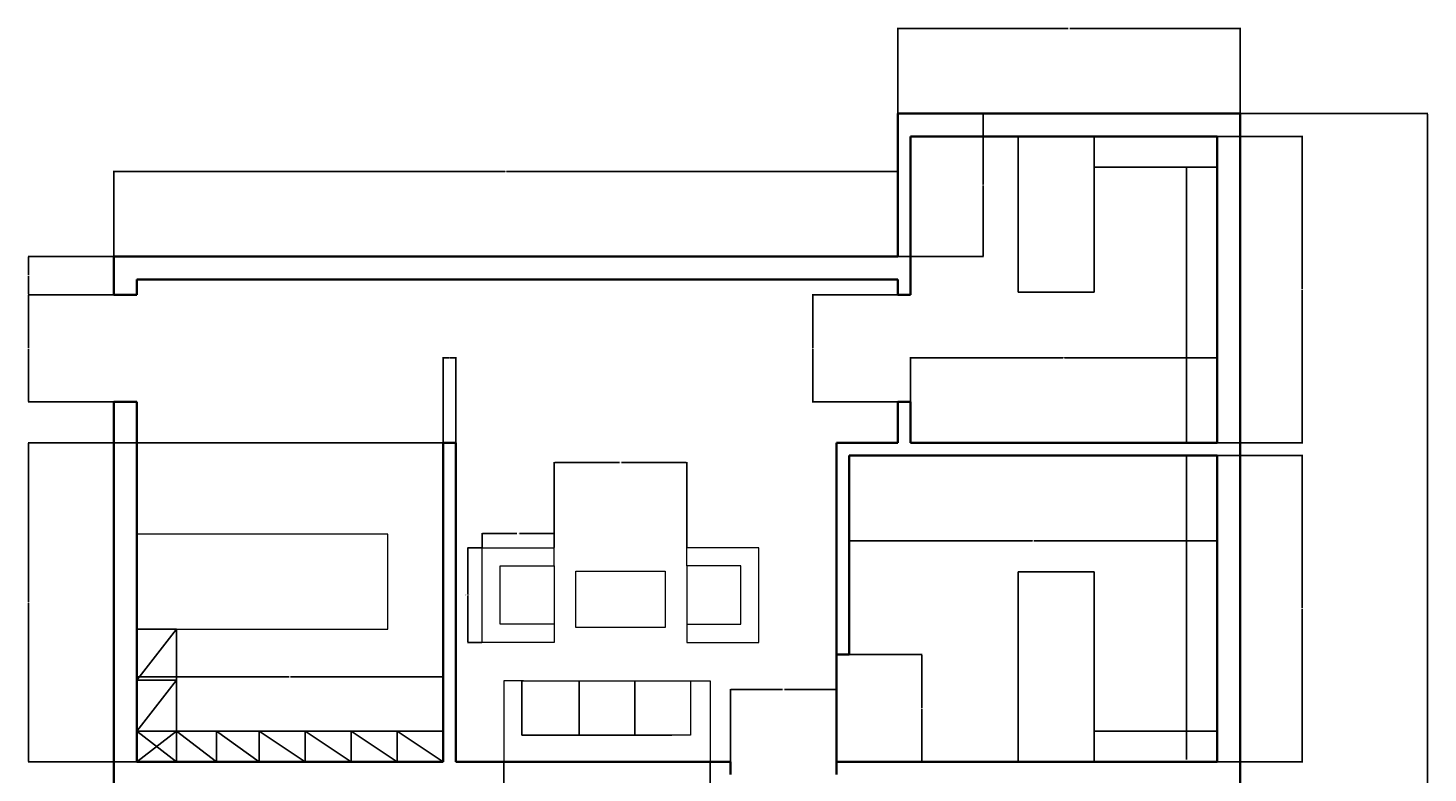
# Model space of a CAD drawing. Units: inches. Extents: x 1201 to 1750, y 1179 to 1858.
# Tile 3 of 3: x 1201 to 1750, y 1566 to 1858. Entities that reach past the tile are written whole.
import ezdxf

# ---------------------------------------------------------------- set-up
doc = ezdxf.new("R2010")
doc.units = ezdxf.units.IN
for name, color, linetype, lineweight in [('A-ANNO-DIMS', 2, 'Continuous', 18), ('A-FLOR-CASE', 9, 'Continuous', 25), ('A-FURN', 8, 'Continuous', 18), ('A-WALL', 7, 'Continuous', 35)]:
    doc.layers.add(name, color=color, linetype=linetype, lineweight=lineweight)
doc.styles.get("Standard").update_dxf_attribs({"font": 'times.ttf'})
doc.dimstyles.get("Standard").update_dxf_attribs({"dimtxt": 0.18, "dimasz": 0.18, "dimexe": 0.18, "dimexo": 0.0625, "dimgap": 0.09, "dimtad": 0, "dimtih": 1, "dimtoh": 1, "dimdec": 4, "dimzin": 0, "dimdsep": 46, "dimtxsty": 'Standard', "dimcen": 0.09, "dimadec": 0, "dimazin": 0, "dimtfac": 1, "dimtdec": 4, "dimtofl": 0, "dimtmove": 0, "dimatfit": 3, "dimfxl": 1, "dimtolj": 1, "dimtzin": 0, "dimarcsym": 0})

# ---------------------------------------------------------------- blocks, each defined once
blk = doc.blocks.new('CHAIR-LOUNGE')
for p, q in [((28.26, 30.01), (28.26, 37.09)), ((28.26, 7.07), (28.26, 0))]:
    blk.add_line(p, q)
blk.add_lwpolyline([(28.26, 0), (0, 0), (0, 37.09), (28.26, 37.09)])
blk.add_lwpolyline([(7.07, 30.01), (28.26, 30.01), (28.26, 7.07), (7.07, 7.07)], close=True)
blk = doc.blocks.new('*D3')
at = {"layer": 'A-ANNO-DIMS', "color": 0, "lineweight": -2, "transparency": 16777216}
for p, q in [((1379.13, 1654.15), (1373.45, 1654.15)), ((1373.63, 1653.97), (1373.63, 1635.79)), ((1373.63, 1617.24), (1373.63, 1635.43)), ((1379.13, 1617.06), (1373.45, 1617.06))]:
    blk.add_line(p, q, dxfattribs=at)
at = {"layer": 'A-ANNO-DIMS', "color": 0, "transparency": 16777216}
for points in [[(1373.6, 1653.97), (1373.66, 1653.97), (1373.63, 1654.15)], [(1373.6, 1617.24), (1373.66, 1617.24), (1373.63, 1617.06)]]:
    blk.add_solid(points, dxfattribs=at)
at = {"layer": 'Defpoints', "color": 0, "transparency": 16777216}
for p in [(1373.63, 1654.15), (1379.19, 1654.15), (1379.19, 1617.06)]:
    blk.add_point(p, dxfattribs=at)
at = {"layer": 'A-ANNO-DIMS', "color": 0, "transparency": 16777216, "insert": (1373.63, 1635.61), "char_height": 0.18, "attachment_point": 5}
blk.add_mtext('\\A1;LOUNGE CHAIR 37 TYP.', dxfattribs=at)
blk = doc.blocks.new('*D4')
at = {"layer": 'A-ANNO-DIMS', "color": 0, "lineweight": -2, "transparency": 16777216}
for p, q in [((1379.19, 1654.21), (1379.19, 1659.89)), ((1379.37, 1659.71), (1392.8, 1659.71)), ((1407.28, 1659.71), (1393.85, 1659.71)), ((1407.46, 1654.21), (1407.46, 1659.89))]:
    blk.add_line(p, q, dxfattribs=at)
at = {"layer": 'A-ANNO-DIMS', "color": 0, "transparency": 16777216}
for points in [[(1379.37, 1659.74), (1379.37, 1659.68), (1379.19, 1659.71)], [(1407.28, 1659.74), (1407.28, 1659.68), (1407.46, 1659.71)]]:
    blk.add_solid(points, dxfattribs=at)
at = {"layer": 'Defpoints', "color": 0, "transparency": 16777216}
for p in [(1407.46, 1659.71), (1379.19, 1654.15), (1407.46, 1654.15)]:
    blk.add_point(p, dxfattribs=at)
at = {"layer": 'A-ANNO-DIMS', "color": 0, "transparency": 16777216, "insert": (1393.32, 1659.71), "char_height": 0.18, "attachment_point": 5}
blk.add_mtext('\\A1;28 TYP.', dxfattribs=at)
blk = doc.blocks.new('*D8')
at = {"layer": 'A-ANNO-DIMS', "color": 0, "lineweight": -2, "transparency": 16777216}
for p, q in [((1676.05, 1824.24), (1749.52, 1824.24)), ((1749.34, 1824.06), (1749.34, 1518.42)), ((1749.34, 1212.42), (1749.34, 1518.06)), ((1716.05, 1212.24), (1749.52, 1212.24))]:
    blk.add_line(p, q, dxfattribs=at)
at = {"layer": 'A-ANNO-DIMS', "color": 0, "transparency": 16777216}
for points in [[(1749.31, 1824.06), (1749.37, 1824.06), (1749.34, 1824.24)], [(1749.31, 1212.42), (1749.37, 1212.42), (1749.34, 1212.24)]]:
    blk.add_solid(points, dxfattribs=at)
at = {"layer": 'Defpoints', "color": 0, "transparency": 16777216}
for p in [(1675.99, 1824.24), (1749.34, 1824.24), (1715.99, 1212.24)]:
    blk.add_point(p, dxfattribs=at)
at = {"layer": 'A-ANNO-DIMS', "color": 0, "transparency": 16777216, "insert": (1749.34, 1518.24), "char_height": 0.18, "attachment_point": 5}
blk.add_mtext('\\A1;612', dxfattribs=at)
blk = doc.blocks.new('*D9')
at = {"layer": 'A-ANNO-DIMS', "color": 0, "lineweight": -2, "transparency": 16777216}
for p, q in [((1234.99, 1768.3), (1234.99, 1801.77)), ((1235.17, 1801.59), (1388.21, 1801.59)), ((1541.81, 1801.59), (1388.77, 1801.59)), ((1541.99, 1768.3), (1541.99, 1801.77))]:
    blk.add_line(p, q, dxfattribs=at)
at = {"layer": 'A-ANNO-DIMS', "color": 0, "transparency": 16777216}
for points in [[(1235.17, 1801.62), (1235.17, 1801.56), (1234.99, 1801.59)], [(1541.81, 1801.62), (1541.81, 1801.56), (1541.99, 1801.59)]]:
    blk.add_solid(points, dxfattribs=at)
at = {"layer": 'Defpoints', "color": 0, "transparency": 16777216}
for p in [(1541.99, 1801.59), (1234.99, 1768.24), (1541.99, 1768.24)]:
    blk.add_point(p, dxfattribs=at)
at = {"layer": 'A-ANNO-DIMS', "color": 0, "transparency": 16777216, "insert": (1388.49, 1801.59), "char_height": 0.18, "attachment_point": 5}
blk.add_mtext('\\A1;307', dxfattribs=at)
blk = doc.blocks.new('*D10')
at = {"layer": 'A-ANNO-DIMS', "color": 0, "lineweight": -2, "transparency": 16777216}
for p, q in [((1541.99, 1824.3), (1541.99, 1857.77)), ((1542.17, 1857.59), (1608.72, 1857.59)), ((1675.81, 1857.59), (1609.26, 1857.59)), ((1675.99, 1824.3), (1675.99, 1857.77))]:
    blk.add_line(p, q, dxfattribs=at)
at = {"layer": 'A-ANNO-DIMS', "color": 0, "transparency": 16777216}
for points in [[(1542.17, 1857.62), (1542.17, 1857.56), (1541.99, 1857.59)], [(1675.81, 1857.62), (1675.81, 1857.56), (1675.99, 1857.59)]]:
    blk.add_solid(points, dxfattribs=at)
at = {"layer": 'Defpoints', "color": 0, "transparency": 16777216}
for p in [(1675.99, 1857.59), (1541.99, 1824.24), (1675.99, 1824.24)]:
    blk.add_point(p, dxfattribs=at)
at = {"layer": 'A-ANNO-DIMS', "color": 0, "transparency": 16777216, "insert": (1608.99, 1857.59), "char_height": 0.18, "attachment_point": 5}
blk.add_mtext('\\A1;134', dxfattribs=at)
blk = doc.blocks.new('*D11')
at = {"layer": 'A-ANNO-DIMS', "color": 0, "lineweight": -2, "transparency": 16777216}
for p, q in [((1542.05, 1824.24), (1575.52, 1824.24)), ((1575.34, 1824.06), (1575.34, 1796.42)), ((1575.34, 1768.42), (1575.34, 1796.06)), ((1542.05, 1768.24), (1575.52, 1768.24))]:
    blk.add_line(p, q, dxfattribs=at)
at = {"layer": 'A-ANNO-DIMS', "color": 0, "transparency": 16777216}
for points in [[(1575.31, 1824.06), (1575.37, 1824.06), (1575.34, 1824.24)], [(1575.31, 1768.42), (1575.37, 1768.42), (1575.34, 1768.24)]]:
    blk.add_solid(points, dxfattribs=at)
at = {"layer": 'Defpoints', "color": 0, "transparency": 16777216}
for p in [(1541.99, 1824.24), (1541.99, 1768.24), (1575.34, 1768.24)]:
    blk.add_point(p, dxfattribs=at)
at = {"layer": 'A-ANNO-DIMS', "color": 0, "transparency": 16777216, "insert": (1575.34, 1796.24), "char_height": 0.18, "attachment_point": 5}
blk.add_mtext('\\A1;56', dxfattribs=at)
blk = doc.blocks.new('*D12')
at = {"layer": 'A-ANNO-DIMS', "color": 0, "lineweight": -2, "transparency": 16777216}
for p, q in [((1234.92, 1768.24), (1201.46, 1768.24)), ((1201.64, 1768.06), (1201.64, 1760.92)), ((1201.64, 1753.42), (1201.64, 1760.56)), ((1234.92, 1753.24), (1201.46, 1753.24))]:
    blk.add_line(p, q, dxfattribs=at)
at = {"layer": 'A-ANNO-DIMS', "color": 0, "transparency": 16777216}
for points in [[(1201.61, 1768.06), (1201.67, 1768.06), (1201.64, 1768.24)], [(1201.61, 1753.42), (1201.67, 1753.42), (1201.64, 1753.24)]]:
    blk.add_solid(points, dxfattribs=at)
at = {"layer": 'Defpoints', "color": 0, "transparency": 16777216}
for p in [(1201.64, 1768.24), (1234.99, 1768.24), (1234.99, 1753.24)]:
    blk.add_point(p, dxfattribs=at)
at = {"layer": 'A-ANNO-DIMS', "color": 0, "transparency": 16777216, "insert": (1201.64, 1760.74), "char_height": 0.18, "attachment_point": 5}
blk.add_mtext('\\A1;15', dxfattribs=at)
blk = doc.blocks.new('*D13')
at = {"layer": 'A-ANNO-DIMS', "color": 0, "lineweight": -2, "transparency": 16777216}
for p, q in [((1234.924469, 1753.241877), (1201.456969, 1753.241877)), ((1201.636969, 1753.061877), (1201.636969, 1732.421877)), ((1201.636969, 1711.421877), (1201.636969, 1732.061877)), ((1234.924469, 1711.241877), (1201.456969, 1711.241877))]:
    blk.add_line(p, q, dxfattribs=at)
at = {"layer": 'A-ANNO-DIMS', "color": 0, "transparency": 16777216}
for points in [[(1201.606969, 1753.061877), (1201.666969, 1753.061877), (1201.636969, 1753.241877)], [(1201.606969, 1711.421877), (1201.666969, 1711.421877), (1201.636969, 1711.241877)]]:
    blk.add_solid(points, dxfattribs=at)
at = {"layer": 'Defpoints', "color": 0, "transparency": 16777216}
for p in [(1201.636969, 1753.241877), (1234.986969, 1753.241877), (1234.986969, 1711.241877)]:
    blk.add_point(p, dxfattribs=at)
at = {"layer": 'A-ANNO-DIMS', "color": 0, "transparency": 16777216, "insert": (1201.636969, 1732.241877), "char_height": 0.18, "attachment_point": 5}
blk.add_mtext('\\A1;42', dxfattribs=at)
blk = doc.blocks.new('*D18')
at = {"layer": 'A-ANNO-DIMS', "color": 0, "lineweight": -2, "transparency": 16777216}
for p, q in [((1667.05, 1690.24), (1700.52, 1690.24)), ((1700.34, 1690.06), (1700.34, 1630.42)), ((1700.34, 1570.42), (1700.34, 1630.06)), ((1667.05, 1570.24), (1700.52, 1570.24))]:
    blk.add_line(p, q, dxfattribs=at)
at = {"layer": 'A-ANNO-DIMS', "color": 0, "transparency": 16777216}
for points in [[(1700.31, 1690.06), (1700.37, 1690.06), (1700.34, 1690.24)], [(1700.31, 1570.42), (1700.37, 1570.42), (1700.34, 1570.24)]]:
    blk.add_solid(points, dxfattribs=at)
at = {"layer": 'Defpoints', "color": 0, "transparency": 16777216}
for p in [(1666.99, 1690.24), (1666.99, 1570.24), (1700.34, 1570.24)]:
    blk.add_point(p, dxfattribs=at)
at = {"layer": 'A-ANNO-DIMS', "color": 0, "transparency": 16777216, "insert": (1700.34, 1630.24), "char_height": 0.18, "attachment_point": 5}
blk.add_mtext('\\A1;120', dxfattribs=at)
blk = doc.blocks.new('*D19')
at = {"layer": 'A-ANNO-DIMS', "color": 0, "lineweight": -2, "transparency": 16777216}
for p, q in [((1667.05, 1815.24), (1700.52, 1815.24)), ((1700.34, 1815.06), (1700.34, 1755.42)), ((1700.34, 1695.42), (1700.34, 1755.06)), ((1667.05, 1695.24), (1700.52, 1695.24))]:
    blk.add_line(p, q, dxfattribs=at)
at = {"layer": 'A-ANNO-DIMS', "color": 0, "transparency": 16777216}
for points in [[(1700.31, 1815.06), (1700.37, 1815.06), (1700.34, 1815.24)], [(1700.31, 1695.42), (1700.37, 1695.42), (1700.34, 1695.24)]]:
    blk.add_solid(points, dxfattribs=at)
at = {"layer": 'Defpoints', "color": 0, "transparency": 16777216}
for p in [(1666.99, 1815.24), (1666.99, 1695.24), (1700.34, 1695.24)]:
    blk.add_point(p, dxfattribs=at)
at = {"layer": 'A-ANNO-DIMS', "color": 0, "transparency": 16777216, "insert": (1700.34, 1755.24), "char_height": 0.18, "attachment_point": 5}
blk.add_mtext('\\A1;120', dxfattribs=at)
blk = doc.blocks.new('*D31')
at = {"layer": 'A-ANNO-DIMS', "color": 0, "lineweight": -2, "transparency": 16777216}
for p, q in [((1363.92, 1695.24), (1201.46, 1695.24)), ((1201.64, 1695.06), (1201.64, 1632.92)), ((1201.64, 1570.42), (1201.64, 1632.56)), ((1363.92, 1570.24), (1201.46, 1570.24))]:
    blk.add_line(p, q, dxfattribs=at)
at = {"layer": 'A-ANNO-DIMS', "color": 0, "transparency": 16777216}
for points in [[(1201.61, 1695.06), (1201.67, 1695.06), (1201.64, 1695.24)], [(1201.61, 1570.42), (1201.67, 1570.42), (1201.64, 1570.24)]]:
    blk.add_solid(points, dxfattribs=at)
at = {"layer": 'Defpoints', "color": 0, "transparency": 16777216}
for p in [(1201.64, 1695.24), (1363.99, 1695.24), (1363.99, 1570.24)]:
    blk.add_point(p, dxfattribs=at)
at = {"layer": 'A-ANNO-DIMS', "color": 0, "transparency": 16777216, "insert": (1201.64, 1632.74), "char_height": 0.18, "attachment_point": 5}
blk.add_mtext('\\A1;125', dxfattribs=at)
blk = doc.blocks.new('*D32')
at = {"layer": 'A-ANNO-DIMS', "color": 0, "lineweight": -2, "transparency": 16777216}
for p, q in [((1243.99, 1570.3), (1243.99, 1603.77)), ((1244.17, 1603.59), (1303.72, 1603.59)), ((1363.81, 1603.59), (1304.26, 1603.59)), ((1363.99, 1570.3), (1363.99, 1603.77))]:
    blk.add_line(p, q, dxfattribs=at)
at = {"layer": 'A-ANNO-DIMS', "color": 0, "transparency": 16777216}
for points in [[(1244.17, 1603.62), (1244.17, 1603.56), (1243.99, 1603.59)], [(1363.81, 1603.62), (1363.81, 1603.56), (1363.99, 1603.59)]]:
    blk.add_solid(points, dxfattribs=at)
at = {"layer": 'Defpoints', "color": 0, "transparency": 16777216}
for p in [(1363.99, 1603.59), (1243.99, 1570.24), (1363.99, 1570.24)]:
    blk.add_point(p, dxfattribs=at)
at = {"layer": 'A-ANNO-DIMS', "color": 0, "transparency": 16777216, "insert": (1303.99, 1603.59), "char_height": 0.18, "attachment_point": 5}
blk.add_mtext('\\A1;120', dxfattribs=at)
blk = doc.blocks.new('*D33')
at = {"layer": 'A-ANNO-DIMS', "color": 0, "lineweight": -2, "transparency": 16777216}
for p, q in [((1476.42, 1565.3), (1476.42, 1598.77)), ((1476.6, 1598.59), (1496.82, 1598.59)), ((1517.81, 1598.59), (1497.58, 1598.59)), ((1517.99, 1565.3), (1517.99, 1598.77))]:
    blk.add_line(p, q, dxfattribs=at)
at = {"layer": 'A-ANNO-DIMS', "color": 0, "transparency": 16777216}
for points in [[(1476.6, 1598.62), (1476.6, 1598.56), (1476.42, 1598.59)], [(1517.81, 1598.62), (1517.81, 1598.56), (1517.99, 1598.59)]]:
    blk.add_solid(points, dxfattribs=at)
at = {"layer": 'Defpoints', "color": 0, "transparency": 16777216}
for p in [(1517.99, 1598.59), (1476.42, 1565.24), (1517.99, 1565.24)]:
    blk.add_point(p, dxfattribs=at)
at = {"layer": 'A-ANNO-DIMS', "color": 0, "transparency": 16777216, "insert": (1497.2, 1598.59), "char_height": 0.18, "attachment_point": 5}
blk.add_mtext('\\A1;41.57', dxfattribs=at)
blk = doc.blocks.new('*D34')
at = {"layer": 'A-ANNO-DIMS', "color": 0, "lineweight": -2, "transparency": 16777216}
for p, q in [((1522.99, 1690.18), (1522.99, 1656.71)), ((1666.99, 1690.18), (1666.99, 1656.71)), ((1523.17, 1656.89), (1594.72, 1656.89)), ((1666.81, 1656.89), (1595.26, 1656.89))]:
    blk.add_line(p, q, dxfattribs=at)
at = {"layer": 'A-ANNO-DIMS', "color": 0, "transparency": 16777216}
for points in [[(1523.17, 1656.92), (1523.17, 1656.86), (1522.99, 1656.89)], [(1666.81, 1656.92), (1666.81, 1656.86), (1666.99, 1656.89)]]:
    blk.add_solid(points, dxfattribs=at)
at = {"layer": 'Defpoints', "color": 0, "transparency": 16777216}
for p in [(1522.99, 1690.24), (1666.99, 1690.24), (1522.99, 1656.89)]:
    blk.add_point(p, dxfattribs=at)
at = {"layer": 'A-ANNO-DIMS', "color": 0, "transparency": 16777216, "insert": (1594.99, 1656.89), "char_height": 0.18, "attachment_point": 5}
blk.add_mtext('\\A1;144', dxfattribs=at)
blk = doc.blocks.new('*D35')
at = {"layer": 'A-ANNO-DIMS', "color": 0, "lineweight": -2, "transparency": 16777216}
for p, q in [((1546.99, 1695.3), (1546.99, 1728.77)), ((1547.17, 1728.59), (1606.72, 1728.59)), ((1666.81, 1728.59), (1607.26, 1728.59)), ((1666.99, 1695.3), (1666.99, 1728.77))]:
    blk.add_line(p, q, dxfattribs=at)
at = {"layer": 'A-ANNO-DIMS', "color": 0, "transparency": 16777216}
for points in [[(1547.17, 1728.62), (1547.17, 1728.56), (1546.99, 1728.59)], [(1666.81, 1728.62), (1666.81, 1728.56), (1666.99, 1728.59)]]:
    blk.add_solid(points, dxfattribs=at)
at = {"layer": 'Defpoints', "color": 0, "transparency": 16777216}
for p in [(1666.99, 1728.59), (1546.99, 1695.24), (1666.99, 1695.24)]:
    blk.add_point(p, dxfattribs=at)
at = {"layer": 'A-ANNO-DIMS', "color": 0, "transparency": 16777216, "insert": (1606.99, 1728.59), "char_height": 0.18, "attachment_point": 5}
blk.add_mtext('\\A1;120', dxfattribs=at)
blk = doc.blocks.new('*D48')
at = {"layer": 'A-ANNO-DIMS', "color": 0, "lineweight": -2, "transparency": 16777216}
for p, q in [((1541.924469, 1753.241877), (1508.456969, 1753.241877)), ((1508.636969, 1753.061877), (1508.636969, 1732.421877)), ((1508.636969, 1711.421877), (1508.636969, 1732.061877)), ((1541.924469, 1711.241877), (1508.456969, 1711.241877))]:
    blk.add_line(p, q, dxfattribs=at)
at = {"layer": 'A-ANNO-DIMS', "color": 0, "transparency": 16777216}
for points in [[(1508.606969, 1753.061877), (1508.666969, 1753.061877), (1508.636969, 1753.241877)], [(1508.606969, 1711.421877), (1508.666969, 1711.421877), (1508.636969, 1711.241877)]]:
    blk.add_solid(points, dxfattribs=at)
at = {"layer": 'Defpoints', "color": 0, "transparency": 16777216}
for p in [(1508.636969, 1753.241877), (1541.986969, 1753.241877), (1541.986969, 1711.241877)]:
    blk.add_point(p, dxfattribs=at)
at = {"layer": 'A-ANNO-DIMS', "color": 0, "transparency": 16777216, "insert": (1508.636969, 1732.241877), "char_height": 0.18, "attachment_point": 5}
blk.add_mtext('\\A1;42', dxfattribs=at)
blk = doc.blocks.new('*D49')
at = {"layer": 'A-ANNO-DIMS', "color": 0, "lineweight": -2, "transparency": 16777216}
for p, q in [((1518.049469, 1612.241877), (1551.516969, 1612.241877)), ((1551.336969, 1612.061877), (1551.336969, 1591.421877)), ((1551.336969, 1570.421877), (1551.336969, 1591.061877)), ((1518.049469, 1570.241877), (1551.516969, 1570.241877))]:
    blk.add_line(p, q, dxfattribs=at)
at = {"layer": 'A-ANNO-DIMS', "color": 0, "transparency": 16777216}
for points in [[(1551.306969, 1612.061877), (1551.366969, 1612.061877), (1551.336969, 1612.241877)], [(1551.306969, 1570.421877), (1551.366969, 1570.421877), (1551.336969, 1570.241877)]]:
    blk.add_solid(points, dxfattribs=at)
at = {"layer": 'Defpoints', "color": 0, "transparency": 16777216}
for p in [(1517.986969, 1612.241877), (1517.986969, 1570.241877), (1551.336969, 1570.241877)]:
    blk.add_point(p, dxfattribs=at)
at = {"layer": 'A-ANNO-DIMS', "color": 0, "transparency": 16777216, "insert": (1551.336969, 1591.241877), "char_height": 0.18, "attachment_point": 5}
blk.add_mtext('\\A1;42', dxfattribs=at)
blk = doc.blocks.new('*D58')
at = {"layer": 'A-ANNO-DIMS', "color": 0, "lineweight": -2, "transparency": 16777216}
for p, q in [((1363.99, 1695.3), (1363.99, 1728.77)), ((1364.17, 1728.59), (1366.35, 1728.59)), ((1368.81, 1728.59), (1366.63, 1728.59)), ((1368.99, 1695.3), (1368.99, 1728.77))]:
    blk.add_line(p, q, dxfattribs=at)
at = {"layer": 'A-ANNO-DIMS', "color": 0, "transparency": 16777216}
for points in [[(1364.17, 1728.62), (1364.17, 1728.56), (1363.99, 1728.59)], [(1368.81, 1728.62), (1368.81, 1728.56), (1368.99, 1728.59)]]:
    blk.add_solid(points, dxfattribs=at)
at = {"layer": 'Defpoints', "color": 0, "transparency": 16777216}
for p in [(1368.99, 1728.59), (1363.99, 1695.24), (1368.99, 1695.24)]:
    blk.add_point(p, dxfattribs=at)
at = {"layer": 'A-ANNO-DIMS', "color": 0, "transparency": 16777216, "insert": (1366.49, 1728.59), "char_height": 0.18, "attachment_point": 5}
blk.add_mtext('\\A1;5', dxfattribs=at)
blk = doc.blocks.new('*D61')
at = {"layer": 'A-ANNO-DIMS', "color": 0, "lineweight": -2, "transparency": 16777216}
for p, q in [((1407.46, 1654.21), (1407.46, 1687.68)), ((1407.64, 1687.5), (1433.01, 1687.5)), ((1459.14, 1687.5), (1433.76, 1687.5)), ((1459.32, 1654.21), (1459.32, 1687.68))]:
    blk.add_line(p, q, dxfattribs=at)
at = {"layer": 'A-ANNO-DIMS', "color": 0, "transparency": 16777216}
for points in [[(1407.64, 1687.53), (1407.64, 1687.47), (1407.46, 1687.5)], [(1459.14, 1687.53), (1459.14, 1687.47), (1459.32, 1687.5)]]:
    blk.add_solid(points, dxfattribs=at)
at = {"layer": 'Defpoints', "color": 0, "transparency": 16777216}
for p in [(1459.32, 1687.5), (1407.46, 1654.15), (1459.32, 1654.15)]:
    blk.add_point(p, dxfattribs=at)
at = {"layer": 'A-ANNO-DIMS', "color": 0, "transparency": 16777216, "insert": (1433.39, 1687.5), "char_height": 0.18, "attachment_point": 5}
blk.add_mtext('\\A1;51.86', dxfattribs=at)
blk = doc.blocks.new('*D62')
at = {"layer": 'A-ANNO-DIMS', "color": 0, "lineweight": -2, "transparency": 16777216}
for p, q in [((1387.67, 1570.18), (1387.67, 1536.71)), ((1468.48, 1570.18), (1468.48, 1536.71)), ((1387.85, 1536.89), (1427.71, 1536.89)), ((1468.3, 1536.89), (1428.44, 1536.89))]:
    blk.add_line(p, q, dxfattribs=at)
at = {"layer": 'A-ANNO-DIMS', "color": 0, "transparency": 16777216}
for points in [[(1387.85, 1536.92), (1387.85, 1536.86), (1387.67, 1536.89)], [(1468.3, 1536.92), (1468.3, 1536.86), (1468.48, 1536.89)]]:
    blk.add_solid(points, dxfattribs=at)
at = {"layer": 'Defpoints', "color": 0, "transparency": 16777216}
for p in [(1387.67, 1570.24), (1468.48, 1570.24), (1387.67, 1536.89)]:
    blk.add_point(p, dxfattribs=at)
at = {"layer": 'A-ANNO-DIMS', "color": 0, "transparency": 16777216, "insert": (1428.07, 1536.89), "char_height": 0.18, "attachment_point": 5}
blk.add_mtext('\\A1;80.81', dxfattribs=at)

msp = doc.modelspace()

# ---------------------------------------------------------------- linework, layer by layer
at = {"layer": 'A-FLOR-CASE'}
for p, q in [((1589.1264, 1815.2419), (1589.1264, 1754.2074)), ((1618.8742, 1815.2419), (1618.8742, 1803.2419)), ((1618.8742, 1815.2419), (1618.8742, 1754.2074)), ((1618.8742, 1803.2419), (1666.987, 1803.2419)), ((1654.987, 1695.2419), (1654.987, 1803.2419)), ((1589.1264, 1754.2074), (1618.8742, 1754.2074)), ((1654.987, 1571.1497), (1654.987, 1690.2419)), ((1589.1264, 1644.7234), (1618.8742, 1644.7234)), ((1589.1264, 1644.7234), (1589.1264, 1570.2419)), ((1618.8742, 1644.7234), (1618.8742, 1576.2419)), ((1243.987, 1622.1992), (1259.5151, 1622.1992)), ((1259.5151, 1622.1992), (1243.987, 1602.2206)), ((1259.5151, 1622.1992), (1259.5151, 1570.2419)), ((1243.987, 1602.2206), (1259.5151, 1602.2206)), ((1259.5151, 1602.2206), (1243.987, 1582.2419)), ((1243.987, 1582.2419), (1363.987, 1582.2419)), ((1243.987, 1582.2419), (1259.5151, 1570.2419)), ((1259.5151, 1582.2419), (1243.987, 1570.2419)), ((1259.5151, 1582.2419), (1275.2193, 1570.2419)), ((1275.2193, 1582.2419), (1275.2193, 1570.2419)), ((1275.2193, 1582.2419), (1291.987, 1570.2419)), ((1291.987, 1582.2419), (1291.987, 1570.2419)), ((1291.987, 1582.2419), (1309.987, 1570.2419)), ((1309.987, 1582.2419), (1309.987, 1570.2419)), ((1309.987, 1582.2419), (1327.987, 1570.2419)), ((1327.987, 1582.2419), (1327.987, 1570.2419)), ((1327.987, 1582.2419), (1345.987, 1570.2419)), ((1345.987, 1582.2419), (1345.987, 1570.2419)), ((1345.987, 1582.2419), (1363.987, 1570.2419)), ((1618.8742, 1582.2419), (1666.987, 1582.2419)), ((1618.8742, 1582.2419), (1618.8742, 1570.2419))]:
    msp.add_line(p, q, dxfattribs=at)
at = {"layer": 'A-FURN'}
for p, q in [((1395.3963, 1602.0068), (1387.6681, 1602.0068)), ((1387.6681, 1602.0068), (1387.6681, 1570.2419)), ((1394.7798, 1602.0068), (1394.7798, 1580.6482)), ((1460.7479, 1602.0068), (1468.4762, 1602.0068)), ((1468.4762, 1602.0068), (1468.4762, 1570.2419)), ((1394.7798, 1580.6482), (1453.5551, 1580.6482))]:
    msp.add_line(p, q, dxfattribs=at)
for points in [[(1243.987, 1622.1992), (1342.3189, 1622.1992), (1342.3189, 1659.5052), (1243.987, 1659.5052)], [(1415.8717, 1644.9506), (1450.9031, 1644.9506), (1450.9031, 1622.8952), (1415.8717, 1622.8952)], [(1394.7798, 1602.0068), (1417.1802, 1602.0068), (1417.1802, 1580.6482), (1394.7798, 1580.6482)], [(1417.1802, 1602.0068), (1438.964, 1602.0068), (1438.964, 1580.6482), (1417.1802, 1580.6482)], [(1438.964, 1602.0068), (1460.7479, 1602.0068), (1460.7479, 1580.6482), (1438.964, 1580.6482)]]:
    msp.add_lwpolyline(points, close=True, dxfattribs=at)
at = {"layer": 'A-WALL'}
for p, q in [((1541.987, 1824.2419), (1541.987, 1768.2419)), ((1541.987, 1824.2419), (1675.987, 1824.2419)), ((1675.987, 1695.2419), (1675.987, 1824.2419)), ((1546.987, 1815.2419), (1546.987, 1753.2419)), ((1546.987, 1815.2419), (1666.987, 1815.2419)), ((1666.987, 1695.2419), (1666.987, 1815.2419)), ((1234.987, 1768.2419), (1243.987, 1768.2419)), ((1234.987, 1768.2419), (1243.987, 1768.2419)), ((1234.987, 1768.2419), (1234.987, 1753.2419)), ((1234.987, 1768.2419), (1541.987, 1768.2419)), ((1243.987, 1759.2419), (1243.987, 1753.2419)), ((1243.987, 1759.2419), (1541.987, 1759.2419)), ((1541.987, 1759.2419), (1541.987, 1753.2419)), ((1234.987, 1753.2419), (1243.987, 1753.2419)), ((1541.987, 1753.2419), (1546.987, 1753.2419)), ((1234.987, 1711.2419), (1243.987, 1711.2419)), ((1234.987, 1711.2419), (1234.987, 1222.2419)), ((1243.987, 1711.2419), (1243.987, 1570.2419)), ((1541.987, 1711.2419), (1541.987, 1695.2419)), ((1541.987, 1711.2419), (1546.987, 1711.2419)), ((1546.987, 1711.2419), (1546.987, 1695.2419)), ((1363.987, 1695.2419), (1363.987, 1570.2419)), ((1368.987, 1695.2419), (1363.987, 1695.2419)), ((1363.987, 1695.2419), (1363.987, 1570.2419)), ((1368.987, 1695.2419), (1368.987, 1570.2419)), ((1517.987, 1612.2419), (1517.987, 1695.2419)), ((1517.987, 1695.2419), (1541.987, 1695.2419)), ((1546.987, 1695.2419), (1666.987, 1695.2419)), ((1675.987, 1571.1497), (1675.987, 1695.2419)), ((1522.987, 1612.2419), (1522.987, 1690.2419)), ((1522.987, 1690.2419), (1666.987, 1690.2419)), ((1666.987, 1571.1497), (1666.987, 1690.2419)), ((1517.987, 1612.2419), (1522.987, 1612.2419)), ((1517.987, 1612.2419), (1517.987, 1565.2419)), ((1243.987, 1570.2419), (1363.987, 1570.2419)), ((1368.987, 1570.2419), (1476.4162, 1570.2419)), ((1476.4162, 1567.7419), (1476.4162, 1570.2419)), ((1476.4162, 1570.2419), (1476.4162, 1565.2419)), ((1517.987, 1570.2419), (1517.987, 1566.4846)), ((1517.987, 1570.2419), (1517.987, 1565.2419)), ((1517.987, 1570.2419), (1517.987, 1565.2419)), ((1517.987, 1570.2419), (1666.987, 1570.2419)), ((1666.987, 1571.1497), (1666.987, 1570.2419)), ((1675.987, 1571.1497), (1675.987, 1500.2419))]:
    msp.add_line(p, q, dxfattribs=at)

# ---------------------------------------------------------------- block references
at = {"layer": 'A-FURN'}
msp.add_blockref('CHAIR-LOUNGE', (1379.1927, 1617.0641), dxfattribs=at)
at = {"layer": 'A-FURN', "extrusion": (0, 0, -1), "zscale": -1}
msp.add_blockref('CHAIR-LOUNGE', (-1487.5821, 1617.0641), dxfattribs=at)

# ---------------------------------------------------------------- dimensions: what is measured, and where the dimension line sits
at = {"layer": 'A-ANNO-DIMS'}
for base, p1, p2, override, picture, middle in [((1675.987, 1857.5919), (1541.987, 1824.2419), (1675.987, 1824.2419), {"dimdec": 0, "dimlfac": 1, "dimrnd": 0, "dimzin": 0, "dimdsep": 46, "dimlunit": 2}, '*D10', (1608.987, 1857.5919)), ((1541.987, 1801.5919), (1234.987, 1768.2419), (1541.987, 1768.2419), {"dimdec": 0, "dimlfac": 1, "dimrnd": 0, "dimzin": 0, "dimdsep": 46, "dimlunit": 2}, '*D9', (1388.487, 1801.5919)), ((1368.987, 1728.5919), (1363.987, 1695.2419), (1368.987, 1695.2419), {"dimdec": 0, "dimlfac": 1, "dimrnd": 0, "dimzin": 0, "dimdsep": 46, "dimlunit": 2}, '*D58', (1366.487, 1728.5919)), ((1666.987, 1728.5919), (1546.987, 1695.2419), (1666.987, 1695.2419), {"dimdec": 0, "dimlfac": 1, "dimrnd": 0, "dimzin": 0, "dimdsep": 46, "dimlunit": 2}, '*D35', (1606.987, 1728.5919)), ((1459.3179, 1687.5017), (1407.4569, 1654.1517), (1459.3179, 1654.1517), {"dimdec": 2, "dimlfac": 1, "dimrnd": 0, "dimzin": 0, "dimdsep": 46, "dimlunit": 2}, '*D61', (1433.3874, 1687.5017)), ((1363.987, 1603.5919), (1243.987, 1570.2419), (1363.987, 1570.2419), {"dimdec": 0, "dimlfac": 1, "dimrnd": 0, "dimzin": 0, "dimdsep": 46, "dimlunit": 2}, '*D32', (1303.987, 1603.5919)), ((1517.987, 1598.5919), (1476.4162, 1565.2419), (1517.987, 1565.2419), {"dimdec": 2, "dimlfac": 1, "dimrnd": 0, "dimzin": 0, "dimdsep": 46, "dimlunit": 2}, '*D33', (1497.2016, 1598.5919))]:
    dim = msp.add_linear_dim(base=base, p1=p1, p2=p2, dimstyle='Standard', override=override, dxfattribs=at)
    dim.commit()
    dim.dimension.update_dxf_attribs({"geometry": picture, "text_midpoint": middle})
for base, p1, p2, angle, override, picture, middle in [((1575.337, 1768.2419), (1541.987, 1824.2419), (1541.987, 1768.2419), 270, {"dimdec": 0, "dimlfac": 1, "dimrnd": 0, "dimzin": 0, "dimdsep": 46, "dimlunit": 2}, '*D11', (1575.337, 1796.2419)), ((1749.337, 1824.2419), (1715.987, 1212.2419), (1675.987, 1824.2419), 90, {"dimdec": 0, "dimlfac": 1, "dimrnd": 0, "dimzin": 0, "dimdsep": 46, "dimlunit": 2}, '*D8', (1749.337, 1518.2419)), ((1700.337, 1695.2419), (1666.987, 1815.2419), (1666.987, 1695.2419), 270, {"dimdec": 0, "dimlfac": 1, "dimrnd": 0, "dimzin": 0, "dimdsep": 46, "dimlunit": 2}, '*D19', (1700.337, 1755.2419)), ((1201.637, 1768.2419), (1234.987, 1753.2419), (1234.987, 1768.2419), 90, {"dimdec": 0, "dimlfac": 1, "dimrnd": 0, "dimzin": 0, "dimdsep": 46, "dimlunit": 2}, '*D12', (1201.637, 1760.7419)), ((1201.637, 1753.2419), (1234.987, 1711.2419), (1234.987, 1753.2419), 90, {"dimdec": 0, "dimlfac": 1, "dimrnd": 0, "dimzin": 0, "dimdsep": 46, "dimlunit": 2}, '*D13', (1201.637, 1732.2419)), ((1508.637, 1753.2419), (1541.987, 1711.2419), (1541.987, 1753.2419), 90, {"dimdec": 0, "dimlfac": 1, "dimrnd": 0, "dimzin": 0, "dimdsep": 46, "dimlunit": 2}, '*D48', (1508.637, 1732.2419)), ((1201.637, 1695.2419), (1363.987, 1570.2419), (1363.987, 1695.2419), 90, {"dimdec": 0, "dimlfac": 1, "dimrnd": 0, "dimzin": 0, "dimdsep": 46, "dimlunit": 2}, '*D31', (1201.637, 1632.7419)), ((1522.987, 1656.8919), (1666.987, 1690.2419), (1522.987, 1690.2419), 180, {"dimdec": 0, "dimlfac": 1, "dimrnd": 0, "dimzin": 0, "dimdsep": 46, "dimlunit": 2}, '*D34', (1594.987, 1656.8919)), ((1700.337, 1570.2419), (1666.987, 1690.2419), (1666.987, 1570.2419), 270, {"dimdec": 0, "dimlfac": 1, "dimrnd": 0, "dimzin": 0, "dimdsep": 46, "dimlunit": 2}, '*D18', (1700.337, 1630.2419)), ((1551.337, 1570.2419), (1517.987, 1612.2419), (1517.987, 1570.2419), 270, {"dimdec": 0, "dimlfac": 1, "dimrnd": 0, "dimzin": 0, "dimdsep": 46, "dimlunit": 2}, '*D49', (1551.337, 1591.2419)), ((1387.6681, 1536.8919), (1468.4762, 1570.2419), (1387.6681, 1570.2419), 180, {"dimdec": 2, "dimlfac": 1, "dimrnd": 0, "dimzin": 0, "dimdsep": 46, "dimlunit": 2}, '*D62', (1428.0721, 1536.8919))]:
    dim = msp.add_linear_dim(base=base, p1=p1, p2=p2, angle=angle, dimstyle='Standard', override=override, dxfattribs=at)
    dim.commit()
    dim.dimension.update_dxf_attribs({"geometry": picture, "text_midpoint": middle})
dim = msp.add_linear_dim(base=(1407.4569, 1659.7148), p1=(1379.1927, 1654.1517), p2=(1407.4569, 1654.1517), text='<> TYP.', dimstyle='Standard', override={"dimdec": 0, "dimlfac": 1, "dimrnd": 0, "dimzin": 0, "dimdsep": 46, "dimlunit": 2}, dxfattribs=at)
dim.commit()
dim.dimension.update_dxf_attribs({"geometry": '*D4', "text_midpoint": (1393.3248, 1659.7148)})
dim = msp.add_linear_dim(base=(1373.6296, 1654.1517), p1=(1379.1927, 1617.0641), p2=(1379.1927, 1654.1517), angle=90, text='LOUNGE CHAIR <> TYP.', dimstyle='Standard', override={"dimdec": 0, "dimlfac": 1, "dimrnd": 0, "dimzin": 0, "dimdsep": 46, "dimlunit": 2}, dxfattribs=at)
dim.commit()
dim.dimension.update_dxf_attribs({"geometry": '*D3', "text_midpoint": (1373.6296, 1635.6079)})

doc.saveas('drawing.dxf')
